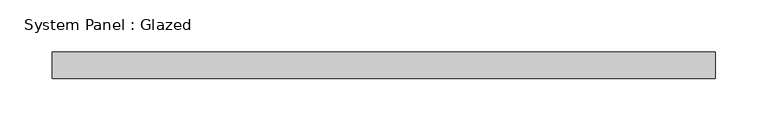
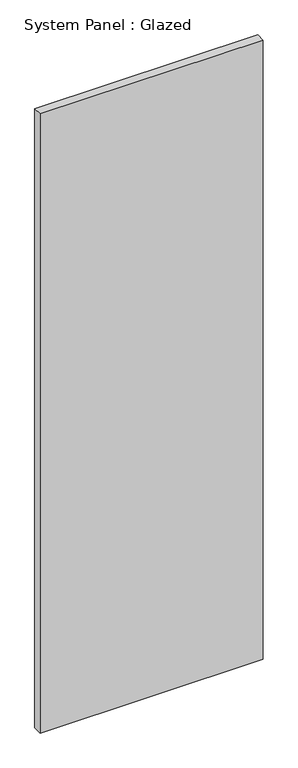
"""IFC4 building model written with IfcOpenShell, lengths in millimetres: plate geometry, System Panel : Glazed."""

from ifc_helpers import new_model, si_unit, origin, origin_with_axes, place, context, project, spatial, polyline, outline, extrude, source, transform, mapped, element, save


def system_panel_glazed_e19ac2e9(model_context):
    return source(origin(), model_context, "Body", "SweptSolid", [
        extrude(outline(polyline([(317.5, 19.05), (-317.5, 19.05), (-317.5, 44.45), (317.5, 44.45), (317.5, 19.05)])), origin_with_axes(), (0.0, 0.0, 1.0), 1861.3028629),
    ])


if __name__ == "__main__":
    model = new_model("IFC4")
    model_context = context("Model", 3, world=origin())
    ifc_project = project(units=[si_unit("LENGTHUNIT", "METRE", prefix="MILLI")], contexts=[model_context])
    site = spatial("IfcSite", under=ifc_project)
    building = spatial("IfcBuilding", under=site)
    placement = place(None, origin())
    system_panel_glazed_shape = system_panel_glazed_e19ac2e9(model_context)
    element("IfcPlate", 1, ObjectType="System Panel : Glazed", at=placement, inside=building, context=model_context, shape_type="MappedRepresentation", body=[
        mapped(system_panel_glazed_shape, transform((0.0, 0.0, 0.0), x_axis=(1.0, 0.0, 0.0), y_axis=(0.0, 1.0, 0.0), z_axis=(0.0, 0.0, 1.0))),
    ])
    save(model, "model.ifc")

# Revit data of these elements
# Type "System Panel : Glazed"
#   Construction Type Id = "GSP4R"
#   Analytic Construction = "1/8 in Pilkington single glazing"
#   Visual Light Transmittance = 0.9
#   Solar Heat Gain Coefficient = 0.86
#   Heat Transfer Coefficient (U) = 1.18115 BTU/(h·ft²·°F)
#   Define Thermal Properties by = 1
# Element 1 (IfcPlate, "System Panel : Glazed")
#   Materials on its faces: "Glass"
# Materials
#   "Glass": class "Glass", colour RGB 0 128 192, transparency 0.75, Description = "Soda Lime Glass", Cost = 0
